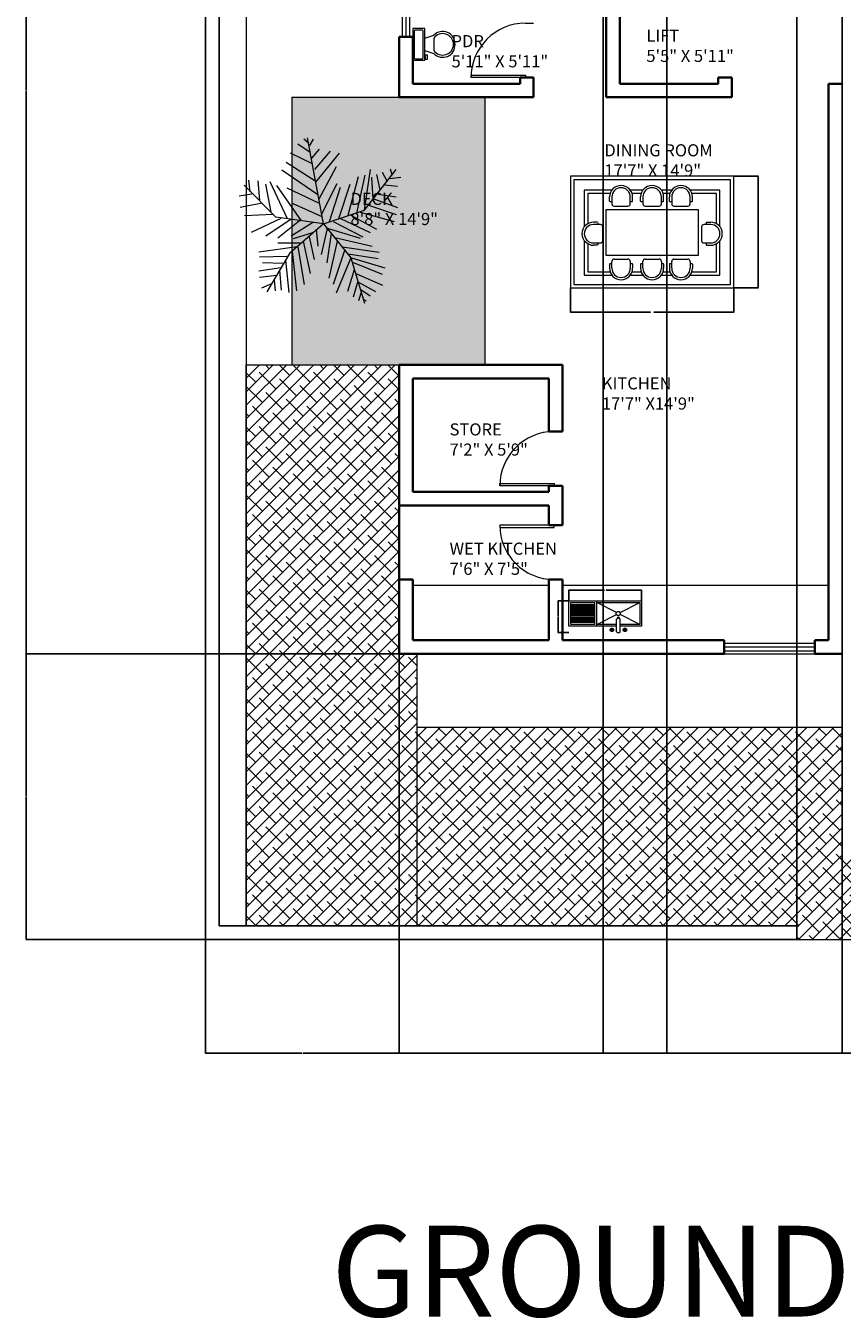
# Model space of a CAD drawing. Units: inches. Extents: x -4843 to -3402, y -164 to 3629.
# Tile 1 of 22: x -4843 to -4303, y -164 to 691. Entities that reach past the tile are written whole.
import ezdxf

# ---------------------------------------------------------------- set-up
doc = ezdxf.new("R2010")
doc.units = ezdxf.units.IN
for name, color, linetype, lineweight in [('A-ANNO-DIMS', 2, 'Continuous', 18), ('A-ANNO-TEXT', 7, 'Continuous', 25), ('A-AREA-IDEN', 2, 'Continuous', 18), ('A-FLOR-CASE', 7, 'Continuous', 18), ('A-FLOR-DECK', 7, 'Continuous', 18), ('C-PROP', 7, 'Continuous', 25), ('C-PVMT', 7, 'Continuous', 18), ('doors', 2, 'Continuous', 18), ('furniture', 6, 'Continuous', 18), ('kitchen', 40, 'Continuous', 18), ('L-PLNT-EDGE', 7, 'Continuous', 18), ('PLANTS', 3, 'Continuous', 13), ('toilets', 5, 'Continuous', 18), ('walls', 7, 'Continuous', 35), ('windows', 1, 'Continuous', 18)]:
    doc.layers.add(name, color=color, linetype=linetype, lineweight=lineweight)
doc.layers.add('A-FLOR-PATT', color=30, linetype='Continuous', lineweight=13, true_color=0xf26722)
doc.layers.add('C-PVMT-PATT', color=9, linetype='Continuous', lineweight=13, true_color=0xc7c8ca)
doc.styles.get("Standard").update_dxf_attribs({"font": 'arial.ttf'})
doc.dimstyles.get("Standard").update_dxf_attribs({"dimtxt": 0.18, "dimasz": 0.18, "dimexe": 0.18, "dimexo": 0.0625, "dimgap": 0.09, "dimtad": 0, "dimtih": 1, "dimtoh": 1, "dimdec": 4, "dimzin": 0, "dimdsep": 46, "dimtxsty": 'Standard', "dimcen": 0.09, "dimadec": 0, "dimazin": 0, "dimtfac": 1, "dimtdec": 4, "dimtofl": 0, "dimtmove": 0, "dimatfit": 3, "dimfxl": 1, "dimtolj": 1, "dimtzin": 0, "dimarcsym": 0})

# ---------------------------------------------------------------- blocks, each defined once
blk = doc.blocks.new('windw 3')
at = {"layer": 'windows'}
for p, q in [((0, 7), (36, 7)), ((0, 4.5), (36, 4.5)), ((0, 2), (36, 2))]:
    blk.add_line(p, q, dxfattribs=at)
for points in [[(0, 0), (0, 9)], [(36, 9), (36, 0)]]:
    blk.add_lwpolyline(points, dxfattribs=at)
blk = doc.blocks.new('window')
at = {"layer": 'windows'}
for p, q in [((0, 7), (60, 7)), ((0, 4.5), (60, 4.5)), ((0, 2), (60, 2))]:
    blk.add_line(p, q, dxfattribs=at)
for points in [[(0, 9), (0, 0)], [(60, 0), (60, 9)]]:
    blk.add_lwpolyline(points, dxfattribs=at)
blk = doc.blocks.new('*U8')
for p, q in [((0, 0), (0, -6)), ((-40, 0), (-40, -6))]:
    blk.add_line(p, q)
blk.add_lwpolyline([(0, 0), (0, 40), (-1.75, 40), (-1.75, 0)], close=True)
blk.add_arc((0, 0), 40, 90, 180)
blk = doc.blocks.new('*U7')
for p, q in [((0, 0), (0, -6)), ((40, 0), (40, -6))]:
    blk.add_line(p, q)
blk.add_lwpolyline([(0, 0), (0, 40), (1.75, 40), (1.75, 0)], close=True)
blk.add_arc((0, 0), 40, 0, 90)
blk = doc.blocks.new('A$C694E1FEF')
for p, q in [((276, 533), (322, 505)), ((313, 542), (284, 496)), ((384, 557), (384, 329)), ((447, 557), (447, 329)), ((505, 514), (559, 524)), ((527, 546), (537, 492)), ((31, 31), (31, 422)), ((31, 422), (385, 243)), ((31, 422), (384, 422)), ((447, 422), (804, 422)), ((804, 422), (451, 243)), ((804, 453), (804, 0)), ((836, 422), (1270, 422)), ((836, 422), (836, 31)), ((836, 390), (1270, 390)), ((1270, 378), (836, 378)), ((836, 359), (1270, 359)), ((1270, 346), (836, 346)), ((836, 327), (1270, 327)), ((1270, 315), (836, 315)), ((836, 296), (1270, 296)), ((1270, 283), (836, 283)), ((836, 264), (1270, 264)), ((1270, 252), (836, 252)), ((836, 233), (1270, 233)), ((1270, 422), (1270, 31)), ((385, 210), (31, 31)), ((804, 31), (31, 31)), ((451, 210), (804, 31)), ((1270, 220), (836, 220)), ((836, 201), (1270, 201)), ((1270, 189), (836, 189)), ((836, 170), (1270, 170)), ((1270, 157), (836, 157)), ((836, 138), (1270, 138)), ((1270, 126), (836, 126)), ((836, 107), (1270, 107)), ((1270, 94), (836, 94)), ((836, 75), (1270, 75)), ((1270, 63), (836, 63)), ((1270, 31), (836, 31))]:
    blk.add_line(p, q)
blk.add_lwpolyline([(447, 453), (1302, 453), (1302, 0), (0, 0), (0, 453), (384, 453)])
for points in [[(329, 519), (329, 527), (321, 541), (307, 549), (290, 549), (276, 541), (268, 527), (268, 511), (276, 497), (290, 489), (307, 489), (321, 497), (329, 511), (329, 519)], [(326, 519), (326, 526), (318, 539), (306, 546), (291, 546), (279, 539), (272, 526), (272, 512), (279, 499), (291, 492), (306, 492), (318, 499), (326, 512), (326, 519)], [(447, 557), (438, 565), (415, 570), (393, 565), (384, 557)], [(562, 519), (562, 527), (554, 541), (540, 549), (524, 549), (510, 541), (502, 527), (502, 511), (510, 497), (524, 489), (540, 489), (554, 497), (562, 511), (562, 519)], [(559, 519), (559, 526), (552, 539), (539, 546), (525, 546), (512, 539), (505, 526), (505, 512), (512, 499), (525, 492), (539, 492), (552, 499), (559, 512), (559, 519)], [(455, 227), (455, 236), (445, 253), (428, 263), (408, 263), (391, 253), (381, 236), (381, 217), (391, 200), (408, 190), (428, 190), (445, 200), (455, 217), (455, 227)], [(384, 329), (389, 321), (406, 312), (425, 312), (442, 321), (447, 329)], [(392, 321), (391, 314), (397, 302), (408, 294), (422, 294), (434, 302), (440, 314), (439, 321)], [(395, 319), (395, 313), (400, 303), (410, 297), (421, 297), (431, 303), (436, 313), (436, 319)]]:
    blk.add_open_spline(points, degree=2)
blk = doc.blocks.new('A$C27801A2F')
for p, q in [((3.55, 2.425), (0, 2.425)), ((0, 2.425), (0, 0)), ((3.475, 2.35), (0.075, 2.35)), ((0.075, 2.35), (0.075, 0.075)), ((3.475, 0.075), (3.475, 2.35)), ((3.55, 0), (3.55, 2.425)), ((0.9, 2.125), (0.3, 2.125)), ((0.3, 2.125), (0.3, 1.325)), ((0.375, 2.05), (0.375, 1.392)), ((0.862, 2.05), (0.375, 2.05)), ((0.85, 1.885), (0.85, 1.975)), ((0.9, 1.975), (0.9, 1.825)), ((1.575, 2.125), (1.3, 2.125)), ((1.3, 1.825), (1.3, 1.975)), ((1.537, 2.05), (1.338, 2.05)), ((1.35, 1.885), (1.35, 1.975)), ((1.525, 1.885), (1.525, 1.975)), ((1.575, 1.975), (1.575, 1.825)), ((2.2, 2.125), (1.975, 2.125)), ((1.975, 1.825), (1.975, 1.975)), ((2.162, 2.05), (2.013, 2.05)), ((2.025, 1.885), (2.025, 1.975)), ((2.15, 1.885), (2.15, 1.975)), ((2.2, 1.975), (2.2, 1.825)), ((3.25, 2.125), (2.6, 2.125)), ((2.6, 1.825), (2.6, 1.975)), ((3.175, 2.05), (2.638, 2.05)), ((2.65, 1.885), (2.65, 1.975)), ((3.175, 1.392), (3.175, 2.05)), ((3.25, 1.325), (3.25, 2.125)), ((0.775, 0.7), (0.775, 1.7)), ((0.775, 1.7), (2.775, 1.7)), ((0.86, 1.875), (0.9, 1.875)), ((0.95, 1.775), (1.25, 1.775)), ((1.3, 1.875), (1.34, 1.875)), ((1.535, 1.875), (1.575, 1.875)), ((1.625, 1.775), (1.925, 1.775)), ((1.975, 1.875), (2.015, 1.875)), ((2.16, 1.875), (2.2, 1.875)), ((2.25, 1.775), (2.55, 1.775)), ((2.6, 1.875), (2.64, 1.875)), ((2.775, 1.7), (2.775, 0.7)), ((0.59, 1.425), (0.5, 1.425)), ((0.6, 1.375), (0.6, 1.415)), ((2.95, 1.415), (2.95, 1.375)), ((2.96, 1.425), (3.05, 1.425)), ((0.65, 1.375), (0.5, 1.375)), ((0.7, 1.025), (0.7, 1.325)), ((2.85, 1.325), (2.85, 1.025)), ((3.05, 1.375), (2.9, 1.375)), ((0.3, 1.025), (0.3, 0.275)), ((0.375, 0.958), (0.375, 0.35)), ((0.5, 0.975), (0.65, 0.975)), ((0.59, 0.925), (0.5, 0.925)), ((0.6, 0.935), (0.6, 0.975)), ((2.9, 0.975), (3.05, 0.975)), ((2.95, 0.975), (2.95, 0.935)), ((2.96, 0.925), (3.05, 0.925)), ((3.175, 0.35), (3.175, 0.958)), ((3.25, 0.275), (3.25, 1.025)), ((2.775, 0.7), (0.775, 0.7)), ((0.9, 0.425), (0.9, 0.575)), ((0.95, 0.625), (1.25, 0.625)), ((1.3, 0.575), (1.3, 0.425)), ((1.575, 0.425), (1.575, 0.575)), ((1.625, 0.625), (1.925, 0.625)), ((1.975, 0.575), (1.975, 0.425)), ((2.2, 0.425), (2.2, 0.575)), ((2.25, 0.625), (2.55, 0.625)), ((2.6, 0.575), (2.6, 0.425)), ((0.375, 0.35), (0.862, 0.35)), ((0.85, 0.515), (0.85, 0.425)), ((0.86, 0.525), (0.9, 0.525)), ((1.3, 0.525), (1.34, 0.525)), ((1.338, 0.35), (1.537, 0.35)), ((1.35, 0.515), (1.35, 0.425)), ((1.525, 0.515), (1.525, 0.425)), ((1.535, 0.525), (1.575, 0.525)), ((1.975, 0.525), (2.015, 0.525)), ((2.013, 0.35), (2.162, 0.35)), ((2.025, 0.515), (2.025, 0.425)), ((2.15, 0.515), (2.15, 0.425)), ((2.16, 0.525), (2.2, 0.525)), ((2.6, 0.525), (2.64, 0.525)), ((2.638, 0.35), (3.175, 0.35)), ((2.65, 0.515), (2.65, 0.425)), ((0, 0), (3.55, 0)), ((0.075, 0.075), (3.475, 0.075)), ((0.3, 0.275), (0.9, 0.275)), ((1.3, 0.275), (1.575, 0.275)), ((1.975, 0.275), (2.2, 0.275)), ((2.6, 0.275), (3.25, 0.275))]:
    blk.add_line(p, q)
for centre, radius, start, end in [((1.1, 1.975), 0.25, 0, 180), ((1.1, 1.975), 0.2, 0.0001, 179.9999), ((1.775, 1.975), 0.25, 0, 180), ((1.775, 1.975), 0.2, 0.0001, 179.9999), ((2.4, 1.975), 0.25, 0, 180), ((2.4, 1.975), 0.2, 0.0001, 179.9999), ((0.86, 1.885), 0.01, 180, 270), ((0.95, 1.825), 0.05, 180, 270), ((1.25, 1.825), 0.05, 270, 0), ((1.34, 1.885), 0.01, 270, 0), ((1.535, 1.885), 0.01, 180, 270), ((1.625, 1.825), 0.05, 180, 270), ((1.925, 1.825), 0.05, 270, 0), ((2.015, 1.885), 0.01, 270, 0), ((2.16, 1.885), 0.01, 180, 270), ((2.25, 1.825), 0.05, 180, 270), ((2.55, 1.825), 0.05, 270, 0), ((2.64, 1.885), 0.01, 270, 0), ((0.5, 1.175), 0.25, 90, 270), ((2.96, 1.415), 0.01, 90, 180), ((3.05, 1.175), 0.25, 270, 90), ((0.5, 1.175), 0.2, 90.0001, 269.9999), ((0.65, 1.325), 0.05, 0, 90), ((2.9, 1.325), 0.05, 90, 180), ((3.05, 1.175), 0.2, 270.0001, 89.9999), ((0.65, 1.025), 0.05, 270, 0), ((2.9, 1.025), 0.05, 180, 270), ((2.96, 0.935), 0.01, 180, 270), ((0.95, 0.575), 0.05, 90, 180), ((1.25, 0.575), 0.05, 0, 90), ((1.625, 0.575), 0.05, 90, 180), ((1.925, 0.575), 0.05, 0, 90), ((2.25, 0.575), 0.05, 90, 180), ((2.55, 0.575), 0.05, 0, 90), ((0.86, 0.515), 0.01, 90, 180), ((1.1, 0.425), 0.25, 180, 0), ((1.1, 0.425), 0.2, 180.0001, 359.9999), ((1.34, 0.515), 0.01, 0, 90), ((1.535, 0.515), 0.01, 90, 180), ((1.775, 0.425), 0.25, 180, 0), ((1.775, 0.425), 0.2, 180.0001, 359.9999), ((2.015, 0.515), 0.01, 0, 90), ((2.16, 0.515), 0.01, 90, 180), ((2.4, 0.425), 0.25, 180, 0), ((2.4, 0.425), 0.2, 180.0001, 359.9999), ((2.64, 0.515), 0.01, 0, 90)]:
    blk.add_arc(centre, radius, start, end)
blk = doc.blocks.new('*U31')
for p, q in [((-254, -215.9), (-203.2, -215.9)), ((-254, -241.3), (-254, -215.9)), ((-203.2, -215.9), (-203.2, -203.2)), ((-177.8, -203.2), (-177.8, -241.3)), ((-101.6, -203.2), (-152.4, -355.6)), ((101.6, -203.2), (152.4, -355.6)), ((241.3, -152.4), (241.3, -50.8)), ((-177.8, -241.3), (-254, -241.3)), ((101.6, -355.6), (-101.6, -355.6))]:
    blk.add_line(p, q)
blk.add_lwpolyline([(266.7, -203.2), (266.7, 0), (-266.7, 0), (-266.7, -203.2)], close=True)
for points in [[(-241.3, -50.8), (-241.3, -152.4)], [(215.9, -25.4), (-215.9, -25.4)], [(-215.9, -177.8), (215.9, -177.8)]]:
    blk.add_lwpolyline(points)
for centre, radius, start, end in [((-219.075, -47.625), 22.45064, 81.8699, 188.1301), ((-219.075, -155.575), 22.45064, 171.869898, 278.1301), ((219.075, -47.625), 22.45064, 351.8699, 98.1301), ((219.075, -155.575), 22.45064, 261.8699, 8.1301), ((-12.12088, -505.93752), 205.61935, 133.01722, 273.38), ((0.94996, -504.77674), 181.02486, 124.50543, 269.7), ((-0.94742, -504.77674), 181.02486, 270.3, 55.4946), ((12.12342, -505.93752), 205.61935, 266.62, 46.9828)]:
    blk.add_arc(centre, radius, start, end)
blk = doc.blocks.new('*U33')
for p, q in [((-221.9198, 1197.3052), (-433.5526, 1338.8594)), ((-258.7244, 1362.456), (-332.3336, 1421.4348)), ((0, 0), (-266.7, 1447.8)), ((-231.1146, 1315.2628), (-166.7002, 1421.4348)), ((-185.1152, 1008.5578), (-553.1612, 1185.4942)), ((-194.31, 1102.9442), (-65.4812, 1256.284)), ((-148.3106, 914.1968), (118.5418, 1220.9018)), ((-129.8956, 701.8528), (265.7602, 1185.4942)), ((-93.091, 489.5342), (-700.3796, 902.3858)), ((-129.8956, 713.6638), (-626.7704, 1032.1544)), ((-74.7014, 418.7444), (219.7608, 961.39)), ((685.8, 228.6), (1219.2, 914.4)), ((689.0258, 230.0224), (790.2448, 914.1968)), ((1121.4862, 925.9824), (1149.0706, 831.6214)), ((-1234.059, 536.7274), (-1252.4486, 737.2604)), ((-1105.2302, 725.4494), (-1077.6458, 395.1732)), ((-976.4268, 666.4706), (-884.4026, 194.6402)), ((-902.8176, 713.6638), (-617.5756, 100.2538)), ((-28.6766, 171.0436), (228.9556, 678.2816)), ((256.5654, 88.4682), (449.7832, 666.4706)), ((412.9786, 147.447), (587.8068, 796.2392)), ((560.197, 182.8292), (698.2206, 819.8358)), ((808.6344, 784.4282), (827.0494, 418.7444)), ((891.4384, 831.6214), (946.658, 572.1096)), ((983.4626, 867.0036), (1066.2666, 725.4494)), ((1029.462, 654.685), (1241.0948, 631.0884)), ((1112.2914, 760.8316), (1296.3144, 784.4282)), ((-1206.4492, 501.3198), (-1418.082, 465.9376)), ((-800.1, 114.3), (-1333.5, 647.7)), ((-369.1382, 53.086), (-783.1836, 642.874)), ((-617.5756, 607.4918), (-74.7014, 347.98)), ((100.1268, 41.275), (284.1498, 619.2774)), ((919.0482, 501.3198), (1222.6798, 454.152)), ((-1031.621, 347.98), (-1399.667, 277.1902)), ((-525.5514, 347.98), (-28.6766, 123.8504)), ((0, 0), (685.8, 228.6)), ((753.4148, 312.5978), (1222.6798, 159.2326)), ((845.439, 418.7444), (1241.0948, 277.1902)), ((-847.598, 159.2326), (-1326.0578, 135.636)), ((-718.7946, 88.4682), (-1215.644, -147.447)), ((-543.9664, 76.6572), (-967.2066, -206.4512)), ((0, 0), (-800.1, 114.3)), ((-405.9428, 53.086), (-764.794, -241.8334)), ((0, 0), (-571.5, -495.3)), ((-166.7002, 29.4894), (-543.9664, -206.4512)), ((0, 0), (457.2, -571.5)), ((164.5412, 41.275), (661.416, -218.2368)), ((284.1498, 88.4682), (781.0246, -147.447)), ((458.978, 147.447), (891.4384, -88.4682)), ((615.4166, 194.6402), (1185.8752, 41.275)), ((-166.7002, -147.447), (-507.1618, -253.619)), ((-120.7008, -88.4682), (-93.091, -371.5766)), ((63.3222, -76.6826), (-37.8714, -513.1308)), ((44.9326, -64.897), (615.4166, -241.8334)), ((127.7366, -159.258), (54.1274, -654.685)), ((-442.7474, -383.3876), (-1086.8406, -477.7486)), ((-387.5278, -324.4088), (-764.794, -324.4088)), ((-433.5526, -383.3876), (-323.1134, -1020.3688)), ((-341.5284, -289.0012), (-221.9198, -831.6214)), ((-240.3094, -218.2368), (-157.5054, -595.7062)), ((228.9556, -289.0012), (90.932, -914.1968)), ((357.759, -430.5554), (164.5412, -1020.3688)), ((192.151, -230.0224), (817.8292, -371.5766)), ((311.7596, -383.3876), (937.4378, -477.7486)), ((-617.5756, -548.5384), (-1077.6458, -560.324)), ((-571.5, -495.3), (-952.5, -1143)), ((-635.9652, -607.5172), (-580.771, -1150.1374)), ((-525.5514, -465.963), (-451.9422, -1126.5408)), ((458.978, -572.1096), (210.5406, -1161.923)), ((412.9786, -501.3452), (919.0482, -583.9206)), ((457.2, -571.5), (685.8, -1333.5)), ((468.1982, -572.1096), (1029.462, -737.2604)), ((486.5878, -642.8994), (983.4626, -843.4324)), ((-718.7946, -737.2604), (-1086.8406, -796.2392)), ((-783.1836, -867.029), (-1077.6458, -902.4112)), ((-681.9646, -666.496), (-1022.4262, -654.685)), ((-737.1842, -784.4536), (-709.5744, -1114.7298)), ((514.1976, -772.6426), (403.7838, -1138.3264)), ((541.8074, -831.6214), (992.6574, -1032.1544)), ((-875.2078, -1008.5832), (-1040.8412, -1079.3476)), ((-829.2084, -937.7934), (-810.7934, -1126.5408)), ((578.612, -961.39), (495.7826, -1232.7128)), ((578.612, -973.1756), (873.0488, -1138.3264)), ((624.6114, -1161.923), (587.8068, -1291.6916)), ((624.6114, -1102.9442), (781.0246, -1209.1162)), ((679.8056, -1268.095), (716.6102, -1291.6916))]:
    blk.add_line(p, q)
blk = doc.blocks.new('*D52')
at = {"layer": 'A-ANNO-DIMS', "color": 0, "lineweight": -2, "transparency": 16777216}
for p, q in [((-4483.42, 310.32), (-4483.42, 317.64)), ((-4483.24, 317.46), (-4459.96, 317.46)), ((-4435.6, 317.46), (-4458.87, 317.46)), ((-4435.42, 310.32), (-4435.42, 317.64))]:
    blk.add_line(p, q, dxfattribs=at)
at = {"layer": 'A-ANNO-DIMS', "color": 0, "transparency": 16777216}
for points in [[(-4483.24, 317.49), (-4483.24, 317.43), (-4483.42, 317.46)], [(-4435.6, 317.49), (-4435.6, 317.43), (-4435.42, 317.46)]]:
    blk.add_solid(points, dxfattribs=at)
at = {"layer": 'Defpoints', "color": 0, "transparency": 16777216}
for p in [(-4483.42, 317.46), (-4483.42, 310.26), (-4435.42, 310.26)]:
    blk.add_point(p, dxfattribs=at)
at = {"layer": 'A-ANNO-DIMS', "color": 0, "transparency": 16777216, "insert": (-4459.42, 317.46), "char_height": 0.18, "attachment_point": 5}
blk.add_mtext('\\A1;SINK 48', dxfattribs=at)
blk = doc.blocks.new('*D53')
at = {"layer": 'A-ANNO-DIMS', "color": 0, "lineweight": -2, "transparency": 16777216}
for p, q in [((-4483.48, 310.26), (-4490.8, 310.26)), ((-4490.62, 310.08), (-4490.62, 299.95)), ((-4490.62, 289.47), (-4490.62, 299.59)), ((-4483.48, 289.29), (-4490.8, 289.29))]:
    blk.add_line(p, q, dxfattribs=at)
at = {"layer": 'A-ANNO-DIMS', "color": 0, "transparency": 16777216}
for points in [[(-4490.65, 310.08), (-4490.59, 310.08), (-4490.62, 310.26)], [(-4490.65, 289.47), (-4490.59, 289.47), (-4490.62, 289.29)]]:
    blk.add_solid(points, dxfattribs=at)
at = {"layer": 'Defpoints', "color": 0, "transparency": 16777216}
for p in [(-4483.42, 310.26), (-4490.62, 289.29), (-4483.42, 289.29)]:
    blk.add_point(p, dxfattribs=at)
at = {"layer": 'A-ANNO-DIMS', "color": 0, "transparency": 16777216, "insert": (-4490.62, 299.77), "char_height": 0.18, "attachment_point": 5}
blk.add_mtext('\\A1;21', dxfattribs=at)
blk = doc.blocks.new('*D56')
at = {"layer": 'A-ANNO-DIMS', "color": 0, "lineweight": -2, "transparency": 16777216}
for p, q in [((-4482.43, 517.3), (-4482.43, 500.98)), ((-4374.43, 517.3), (-4374.43, 500.98)), ((-4482.25, 501.16), (-4429.47, 501.16)), ((-4374.61, 501.16), (-4427.39, 501.16))]:
    blk.add_line(p, q, dxfattribs=at)
at = {"layer": 'A-ANNO-DIMS', "color": 0, "transparency": 16777216}
for points in [[(-4482.25, 501.19), (-4482.25, 501.13), (-4482.43, 501.16)], [(-4374.61, 501.19), (-4374.61, 501.13), (-4374.43, 501.16)]]:
    blk.add_solid(points, dxfattribs=at)
at = {"layer": 'Defpoints', "color": 0, "transparency": 16777216}
for p in [(-4482.43, 517.36), (-4374.43, 517.36), (-4374.43, 501.16)]:
    blk.add_point(p, dxfattribs=at)
at = {"layer": 'A-ANNO-DIMS', "color": 0, "transparency": 16777216, "insert": (-4428.43, 501.16), "char_height": 0.18, "attachment_point": 5}
blk.add_mtext('\\A1;DINING SET 108', dxfattribs=at)
blk = doc.blocks.new('*D57')
at = {"layer": 'A-ANNO-DIMS', "color": 0, "lineweight": -2, "transparency": 16777216}
for p, q in [((-4374.37, 591.14), (-4358.05, 591.14)), ((-4358.23, 590.96), (-4358.23, 554.43)), ((-4358.23, 517.54), (-4358.23, 554.07)), ((-4374.37, 517.36), (-4358.05, 517.36))]:
    blk.add_line(p, q, dxfattribs=at)
at = {"layer": 'A-ANNO-DIMS', "color": 0, "transparency": 16777216}
for points in [[(-4358.26, 590.96), (-4358.2, 590.96), (-4358.23, 591.14)], [(-4358.26, 517.54), (-4358.2, 517.54), (-4358.23, 517.36)]]:
    blk.add_solid(points, dxfattribs=at)
at = {"layer": 'Defpoints', "color": 0, "transparency": 16777216}
for p in [(-4374.43, 591.14), (-4358.23, 591.14), (-4374.43, 517.36)]:
    blk.add_point(p, dxfattribs=at)
at = {"layer": 'A-ANNO-DIMS', "color": 0, "transparency": 16777216, "insert": (-4358.23, 554.25), "char_height": 0.18, "attachment_point": 5}
blk.add_mtext('\\A1;74', dxfattribs=at)
blk = doc.blocks.new('*D62')
at = {"layer": 'A-ANNO-DIMS', "color": 0, "lineweight": -2, "transparency": 16777216}
for p, q in [((-4595.78, 275.29), (-4595.78, 10.92)), ((-4302.78, 275.29), (-4302.78, 10.92)), ((-4595.6, 11.1), (-4449.57, 11.1)), ((-4302.96, 11.1), (-4448.99, 11.1))]:
    blk.add_line(p, q, dxfattribs=at)
at = {"layer": 'A-ANNO-DIMS', "color": 0, "transparency": 16777216}
for points in [[(-4595.6, 11.13), (-4595.6, 11.07), (-4595.78, 11.1)], [(-4302.96, 11.13), (-4302.96, 11.07), (-4302.78, 11.1)]]:
    blk.add_solid(points, dxfattribs=at)
at = {"layer": 'Defpoints', "color": 0, "transparency": 16777216}
for p in [(-4595.78, 275.35), (-4302.78, 275.35), (-4302.78, 11.1)]:
    blk.add_point(p, dxfattribs=at)
at = {"layer": 'A-ANNO-DIMS', "color": 0, "transparency": 16777216, "insert": (-4449.28, 11.1), "char_height": 0.18, "attachment_point": 5}
blk.add_mtext('\\A1;293', dxfattribs=at)
blk = doc.blocks.new('*D63')
at = {"layer": 'A-ANNO-DIMS', "color": 0, "lineweight": -2, "transparency": 16777216}
for p, q in [((-4083.78, 457.29), (-4083.78, 10.92)), ((-4302.78, 275.29), (-4302.78, 10.92)), ((-4302.6, 11.1), (-4193.57, 11.1)), ((-4083.96, 11.1), (-4192.99, 11.1))]:
    blk.add_line(p, q, dxfattribs=at)
at = {"layer": 'A-ANNO-DIMS', "color": 0, "transparency": 16777216}
for points in [[(-4302.6, 11.13), (-4302.6, 11.07), (-4302.78, 11.1)], [(-4083.96, 11.13), (-4083.96, 11.07), (-4083.78, 11.1)]]:
    blk.add_solid(points, dxfattribs=at)
at = {"layer": 'Defpoints', "color": 0, "transparency": 16777216}
for p in [(-4083.78, 457.35), (-4302.78, 275.35), (-4083.78, 11.1)]:
    blk.add_point(p, dxfattribs=at)
at = {"layer": 'A-ANNO-DIMS', "color": 0, "transparency": 16777216, "insert": (-4193.28, 11.1), "char_height": 0.18, "attachment_point": 5}
blk.add_mtext('\\A1;219', dxfattribs=at)
blk = doc.blocks.new('*D64')
at = {"layer": 'A-ANNO-DIMS', "color": 0, "lineweight": -2, "transparency": 16777216}
for p, q in [((-4595.85, 1020.35), (-4842.55, 1020.35)), ((-4842.37, 1020.17), (-4842.37, 648.04)), ((-4842.37, 275.53), (-4842.37, 647.67)), ((-4595.85, 275.35), (-4842.55, 275.35))]:
    blk.add_line(p, q, dxfattribs=at)
at = {"layer": 'A-ANNO-DIMS', "color": 0, "transparency": 16777216}
for points in [[(-4842.4, 1020.17), (-4842.34, 1020.17), (-4842.37, 1020.35)], [(-4842.4, 275.53), (-4842.34, 275.53), (-4842.37, 275.35)]]:
    blk.add_solid(points, dxfattribs=at)
at = {"layer": 'Defpoints', "color": 0, "transparency": 16777216}
for p in [(-4595.78, 1020.35), (-4842.37, 275.35), (-4595.78, 275.35)]:
    blk.add_point(p, dxfattribs=at)
at = {"layer": 'A-ANNO-DIMS', "color": 0, "transparency": 16777216, "insert": (-4842.37, 647.85), "char_height": 0.18, "attachment_point": 5}
blk.add_mtext('\\A1;745', dxfattribs=at)
blk = doc.blocks.new('*D65')
at = {"layer": 'A-ANNO-DIMS', "color": 0, "lineweight": -2, "transparency": 16777216}
for p, q in [((-4595.78, 275.29), (-4595.78, 10.92)), ((-4723.78, 86.29), (-4723.78, 10.92)), ((-4723.6, 11.1), (-4660.06, 11.1)), ((-4595.96, 11.1), (-4659.5, 11.1))]:
    blk.add_line(p, q, dxfattribs=at)
at = {"layer": 'A-ANNO-DIMS', "color": 0, "transparency": 16777216}
for points in [[(-4723.6, 11.13), (-4723.6, 11.07), (-4723.78, 11.1)], [(-4595.96, 11.13), (-4595.96, 11.07), (-4595.78, 11.1)]]:
    blk.add_solid(points, dxfattribs=at)
at = {"layer": 'Defpoints', "color": 0, "transparency": 16777216}
for p in [(-4595.78, 275.35), (-4723.78, 86.35), (-4595.78, 11.1)]:
    blk.add_point(p, dxfattribs=at)
at = {"layer": 'A-ANNO-DIMS', "color": 0, "transparency": 16777216, "insert": (-4659.78, 11.1), "char_height": 0.18, "attachment_point": 5}
blk.add_mtext('\\A1;128', dxfattribs=at)
blk = doc.blocks.new('*D67')
at = {"layer": 'A-ANNO-DIMS', "color": 0, "lineweight": -2, "transparency": 16777216}
for p, q in [((-4595.85, 275.35), (-4842.55, 275.35)), ((-4842.37, 275.17), (-4842.37, 181.04)), ((-4842.37, 86.53), (-4842.37, 180.67)), ((-4723.85, 86.35), (-4842.55, 86.35))]:
    blk.add_line(p, q, dxfattribs=at)
at = {"layer": 'A-ANNO-DIMS', "color": 0, "transparency": 16777216}
for points in [[(-4842.4, 275.17), (-4842.34, 275.17), (-4842.37, 275.35)], [(-4842.4, 86.53), (-4842.34, 86.53), (-4842.37, 86.35)]]:
    blk.add_solid(points, dxfattribs=at)
at = {"layer": 'Defpoints', "color": 0, "transparency": 16777216}
for p in [(-4595.78, 275.35), (-4842.37, 86.35), (-4723.78, 86.35)]:
    blk.add_point(p, dxfattribs=at)
at = {"layer": 'A-ANNO-DIMS', "color": 0, "transparency": 16777216, "insert": (-4842.37, 180.85), "char_height": 0.18, "attachment_point": 5}
blk.add_mtext('\\A1;189', dxfattribs=at)
blk = doc.blocks.new('*D75')
at = {"layer": 'A-ANNO-DIMS', "color": 0, "lineweight": -2, "transparency": 16777216}
for p, q in [((-4460.78, 819.29), (-4460.78, 10.92)), ((-4418.78, 819.29), (-4418.78, 10.92)), ((-4460.6, 11.1), (-4440, 11.1)), ((-4418.96, 11.1), (-4439.56, 11.1))]:
    blk.add_line(p, q, dxfattribs=at)
at = {"layer": 'A-ANNO-DIMS', "color": 0, "transparency": 16777216}
for points in [[(-4460.6, 11.13), (-4460.6, 11.07), (-4460.78, 11.1)], [(-4418.96, 11.13), (-4418.96, 11.07), (-4418.78, 11.1)]]:
    blk.add_solid(points, dxfattribs=at)
at = {"layer": 'Defpoints', "color": 0, "transparency": 16777216}
for p in [(-4460.78, 819.35), (-4418.78, 819.35), (-4418.78, 11.1)]:
    blk.add_point(p, dxfattribs=at)
at = {"layer": 'A-ANNO-DIMS', "color": 0, "transparency": 16777216, "insert": (-4439.78, 11.1), "char_height": 0.18, "attachment_point": 5}
blk.add_mtext('\\A1;42', dxfattribs=at)
blk = doc.blocks.new('*D76')
at = {"layer": 'A-ANNO-DIMS', "color": 0, "lineweight": -2, "transparency": 16777216}
for p, q in [((-4418.78, 819.29), (-4418.78, 10.92)), ((-4302.78, 819.29), (-4302.78, 10.92)), ((-4418.6, 11.1), (-4361.06, 11.1)), ((-4302.96, 11.1), (-4360.5, 11.1))]:
    blk.add_line(p, q, dxfattribs=at)
at = {"layer": 'A-ANNO-DIMS', "color": 0, "transparency": 16777216}
for points in [[(-4418.6, 11.13), (-4418.6, 11.07), (-4418.78, 11.1)], [(-4302.96, 11.13), (-4302.96, 11.07), (-4302.78, 11.1)]]:
    blk.add_solid(points, dxfattribs=at)
at = {"layer": 'Defpoints', "color": 0, "transparency": 16777216}
for p in [(-4418.78, 819.35), (-4302.78, 819.35), (-4302.78, 11.1)]:
    blk.add_point(p, dxfattribs=at)
at = {"layer": 'A-ANNO-DIMS', "color": 0, "transparency": 16777216, "insert": (-4360.78, 11.1), "char_height": 0.18, "attachment_point": 5}
blk.add_mtext('\\A1;116', dxfattribs=at)
blk = doc.blocks.new('*D81')
at = {"layer": 'A-ANNO-DIMS', "color": 0, "lineweight": -2, "transparency": 16777216}
for p, q in [((-4332.78, 86.42), (-4332.78, 1392.95)), ((-4332.6, 1392.77), (-4168.61, 1392.77)), ((-4003.86, 1392.77), (-4167.86, 1392.77)), ((-4003.68, 86.42), (-4003.68, 1392.95))]:
    blk.add_line(p, q, dxfattribs=at)
at = {"layer": 'A-ANNO-DIMS', "color": 0, "transparency": 16777216}
for points in [[(-4332.6, 1392.8), (-4332.6, 1392.74), (-4332.78, 1392.77)], [(-4003.86, 1392.8), (-4003.86, 1392.74), (-4003.68, 1392.77)]]:
    blk.add_solid(points, dxfattribs=at)
at = {"layer": 'Defpoints', "color": 0, "transparency": 16777216}
for p in [(-4003.68, 1392.77), (-4332.78, 86.35), (-4003.68, 86.35)]:
    blk.add_point(p, dxfattribs=at)
at = {"layer": 'A-ANNO-DIMS', "color": 0, "transparency": 16777216, "insert": (-4168.23, 1392.77), "char_height": 0.18, "attachment_point": 5}
blk.add_mtext('\\A1;329.1', dxfattribs=at)

msp = doc.modelspace()

# ---------------------------------------------------------------- hatches: boundary and pattern name
at = {"layer": 'A-FLOR-PATT', "transparency": 33554472}
h = msp.add_hatch(color=256, dxfattribs=at)
h.dxf.hatch_style = 1
h.paths.add_polyline_path([(-4538.62, 643.09), (-4595.62, 643.09), (-4666.62, 643.09), (-4666.62, 466.09), (-4595.62, 466.09), (-4538.62, 466.09)])
h.paths.add_polyline_path([(-3998.62, 888.09), (-4083.62, 888.09), (-4140.62, 888.09), (-4140.62, 652.09), (-4132.62, 652.09), (-4132.62, 650.09), (-4096.62, 650.09), (-4096.62, 652.09), (-4083.62, 652.09), (-3998.62, 652.09)])
at = {"layer": 'C-PVMT-PATT'}
h = msp.add_hatch(dxfattribs=at)
h.set_pattern_fill('ANSI38', color=256, scale=2)
h.set_pattern_definition([(45, (-7766.296, -1992.247), (-4.490128, 4.490128), []), (135, (-7766.296, -1992.247), (-13.470384, 4.490128), [15.875, -9.525])])
h.paths.add_polyline_path([(-4583.98, 275.35), (-4595.78, 275.35), (-4595.78, 324.35), (-4595.78, 373.35), (-4595.78, 466.35), (-4696.78, 466.35), (-4696.78, 95.35), (-4583.98, 95.35), (-4583.98, 226.6)])
h.paths.add_polyline_path([(-4302.78, 226.6), (-4583.98, 226.6), (-4583.98, 95.35), (-4332.78, 95.35), (-4332.78, 86.35), (-4003.68, 86.35), (-4003.68, 95.35), (-3978.78, 95.35), (-3978.78, 457.35), (-4003.68, 457.35), (-4003.68, 139.54), (-4302.78, 139.54)])

# ---------------------------------------------------------------- linework, layer by layer
at = {"layer": 'A-FLOR-CASE'}
for p, q in [((-4496.78, 320.35), (-4586.78, 320.35)), ((-4311.78, 320.35), (-4487.78, 320.35))]:
    msp.add_line(p, q, dxfattribs=at)
at = {"layer": 'A-FLOR-DECK'}
for p, q in [((-4666.78, 643.35), (-4666.78, 466.35)), ((-4666.78, 643.35), (-4595.78, 643.35)), ((-4538.78, 466.35), (-4538.78, 643.35)), ((-4538.78, 466.35), (-4538.78, 643.35)), ((-4666.78, 466.35), (-4595.78, 466.35))]:
    msp.add_line(p, q, dxfattribs=at)
at = {"layer": 'C-PROP'}
for p, q in [((-4723.78, 1149.35), (-4723.78, 86.35)), ((-4714.78, 1140.35), (-4714.78, 95.35)), ((-4714.78, 95.35), (-4332.78, 95.35)), ((-4332.78, 86.35), (-4332.78, 95.35)), ((-4723.78, 86.35), (-4332.78, 86.35))]:
    msp.add_line(p, q, dxfattribs=at)
at = {"layer": 'C-PVMT'}
for p, q in [((-4583.98, 226.6), (-4583.98, 95.35)), ((-4332.78, 86.35), (-4003.68, 86.35))]:
    msp.add_line(p, q, dxfattribs=at)
for points in [[(-4583.98, 95.35), (-4696.78, 95.35), (-4696.78, 466.35), (-4583.98, 466.35)], [(-4583.98, 275.35), (-4583.98, 226.6)], [(-4583.63, 275.35), (-4302.78, 275.35), (-4302.78, 226.6), (-4583.98, 226.6)]]:
    msp.add_lwpolyline(points, dxfattribs=at)
at = {"layer": 'L-PLNT-EDGE'}
msp.add_line((-4696.78, 1116.35), (-4696.78, 95.35), dxfattribs=at)
at = {"layer": 'walls'}
for p, q in [((-4458.78, 723.35), (-4458.78, 643.35)), ((-4449.78, 723.35), (-4449.78, 652.35)), ((-4595.78, 683.35), (-4595.78, 643.35)), ((-4586.78, 683.35), (-4586.78, 652.35)), ((-4586.78, 652.35), (-4515.78, 652.35)), ((-4515.78, 656.35), (-4515.78, 652.35)), ((-4506.78, 656.35), (-4506.78, 643.35)), ((-4449.78, 652.35), (-4384.78, 652.35)), ((-4384.78, 656.35), (-4384.78, 652.35)), ((-4375.78, 656.35), (-4375.78, 643.35)), ((-4311.78, 652.35), (-4311.78, 284.35)), ((-4302.78, 652.35), (-4311.78, 652.35)), ((-4595.78, 643.35), (-4506.78, 643.35)), ((-4458.78, 643.35), (-4375.78, 643.35)), ((-4487.78, 466.35), (-4595.78, 466.35)), ((-4595.78, 466.35), (-4595.78, 373.35)), ((-4487.78, 422.35), (-4487.78, 466.35)), ((-4496.78, 457.35), (-4586.78, 457.35)), ((-4586.78, 457.35), (-4586.78, 382.35)), ((-4496.78, 422.35), (-4496.78, 457.35)), ((-4496.78, 382.35), (-4496.78, 386.35)), ((-4487.78, 360.35), (-4487.78, 386.35)), ((-4586.78, 382.35), (-4496.78, 382.35)), ((-4586.78, 373.35), (-4595.78, 373.35)), ((-4595.78, 324.35), (-4595.78, 373.35)), ((-4586.78, 373.35), (-4496.78, 373.35)), ((-4496.78, 360.35), (-4496.78, 373.35)), ((-4586.78, 324.35), (-4595.78, 324.35)), ((-4595.78, 324.35), (-4595.78, 275.35)), ((-4586.78, 324.35), (-4586.78, 284.35)), ((-4496.78, 284.35), (-4496.78, 324.35)), ((-4487.78, 284.35), (-4487.78, 324.35)), ((-4496.78, 284.35), (-4586.78, 284.35)), ((-4380.78, 284.35), (-4487.78, 284.35)), ((-4380.78, 284.35), (-4487.78, 284.35)), ((-4380.78, 275.35), (-4380.78, 284.35)), ((-4311.78, 284.35), (-4320.78, 284.35)), ((-4311.78, 284.35), (-4320.78, 284.35)), ((-4320.78, 275.35), (-4320.78, 284.35)), ((-4380.78, 275.35), (-4595.78, 275.35)), ((-4302.78, 275.35), (-4320.78, 275.35))]:
    msp.add_line(p, q, dxfattribs=at)
for points in [[(-4586.78, 683.35), (-4595.78, 683.35)], [(-4506.78, 656.35), (-4515.78, 656.35)], [(-4375.78, 656.35), (-4384.78, 656.35)], [(-4496.78, 422.35), (-4487.78, 422.35)], [(-4487.78, 386.35), (-4496.78, 386.35)], [(-4496.78, 360.35), (-4487.78, 360.35)], [(-4487.78, 324.35), (-4496.78, 324.35)]]:
    msp.add_lwpolyline(points, dxfattribs=at)

# ---------------------------------------------------------------- block references
at = {"layer": 'doors', "xscale": 0.9, "yscale": 0.9, "zscale": 0.9, "rotation": 90}
for name, p in [('*U7', (-4512.18, 656.35)), ('*U7', (-4493.18, 386.35)), ('*U8', (-4493.18, 360.35))]:
    msp.add_blockref(name, p, dxfattribs=at)
at = {"layer": 'furniture', "xscale": 30.42253521127383, "yscale": 30.42253521127383, "zscale": 30.42253521127383}
msp.add_blockref('A$C27801A2F', (-4482.43, 517.36), dxfattribs=at)
at = {"layer": 'kitchen', "xscale": 0.0368764537023914, "yscale": 0.0368764537023914, "zscale": 0.0368764537023914, "rotation": 180}
msp.add_blockref('A$C694E1FEF', (-4435.42, 310.26), dxfattribs=at)
at = {"layer": 'PLANTS', "xscale": 0.0393700787401575, "yscale": 0.0393700787401575, "zscale": 0.0393700787401575}
msp.add_blockref('*U33', (-4645.74, 559.62), dxfattribs=at)
at = {"layer": 'toilets', "xscale": 0.0393700787401575, "yscale": 0.0393700787401575, "zscale": 0.0393700787401575, "rotation": 90}
msp.add_blockref('*U31', (-4586.78, 678.35), dxfattribs=at)
at = {"layer": 'windows', "rotation": 270}
msp.add_blockref('windw 3', (-4595.78, 719.35), dxfattribs=at)
at = {"layer": 'windows'}
msp.add_blockref('window', (-4380.78, 275.35), dxfattribs=at)

# ---------------------------------------------------------------- texts
at = {"layer": 'A-ANNO-TEXT'}
msp.add_text('GROUND FLOOR', height=60, dxfattribs=at).set_placement((-4640.63, -163.06))
at = {"layer": 'A-AREA-IDEN', "char_height": 8, "attachment_point": 1}
for s, width, heights, insert in [('PDR\\P5\'11" X 5\'11"', 66.873, [0], (-4561.07, 684.49)), ('LIFT\\P5\'5" X 5\'11"', 66.873, [0], (-4432.24, 688.07)), ('DINING ROOM\\P17\'7" X 14\'9"', 98.9475, [0], (-4459.99, 612.29)), ('DECK\\P8\'8" X 14\'9"', 66.873, [0], (-4627.89, 580.18)), ('KITCHEN \\P17\'7" X14\'9"', 66.873, [0], (-4461.65, 458.14)), ('STORE \\P7\'2" X 5\'9"', 66.873, [0], (-4562.37, 427.68)), ('WET KITCHEN\\P7\'6" X 7\'5"', 139.7591, [37.02], (-4562.37, 348.82))]:
    msp.add_mtext_dynamic_manual_height_columns(s, width=width, gutter_width=60, heights=heights, dxfattribs=dict(at, insert=insert))

# ---------------------------------------------------------------- dimensions: what is measured, and where the dimension line sits
at = {"layer": 'A-ANNO-DIMS'}
for base, p1, p2, override, picture, middle in [((-4003.68, 1392.77), (-4332.78, 86.35), (-4003.68, 86.35), {"dimdec": 1, "dimlfac": 1, "dimrnd": 0, "dimzin": 0, "dimdsep": 46, "dimlunit": 2}, '*D81', (-4168.23, 1392.77)), ((-4418.78, 11.1), (-4460.78, 819.35), (-4418.78, 819.35), {"dimdec": 0, "dimlfac": 1, "dimrnd": 0, "dimzin": 0, "dimdsep": 46, "dimlunit": 2}, '*D75', (-4439.78, 11.1)), ((-4302.78, 11.1), (-4418.78, 819.35), (-4302.78, 819.35), {"dimdec": 0, "dimlfac": 1, "dimrnd": 0, "dimzin": 0, "dimdsep": 46, "dimlunit": 2}, '*D76', (-4360.78, 11.1)), ((-4083.78, 11.1), (-4302.78, 275.35), (-4083.78, 457.35), {"dimdec": 0, "dimlfac": 1, "dimrnd": 0, "dimzin": 0, "dimdsep": 46, "dimlunit": 2}, '*D63', (-4193.28, 11.1)), ((-4595.78, 11.1), (-4723.78, 86.35), (-4595.78, 275.35), {"dimdec": 0, "dimlfac": 1, "dimrnd": 0, "dimzin": 0, "dimdsep": 46, "dimlunit": 2}, '*D65', (-4659.78, 11.1)), ((-4302.78, 11.1), (-4595.78, 275.35), (-4302.78, 275.35), {"dimdec": 0, "dimlfac": 1, "dimrnd": 0, "dimzin": 0, "dimdsep": 46, "dimlunit": 2}, '*D62', (-4449.28, 11.1))]:
    dim = msp.add_linear_dim(base=base, p1=p1, p2=p2, dimstyle='Standard', override=override, dxfattribs=at)
    dim.commit()
    dim.dimension.update_dxf_attribs({"geometry": picture, "text_midpoint": middle})
for base, p1, p2, angle, picture, middle in [((-4842.37, 275.35), (-4595.78, 1020.35), (-4595.78, 275.35), 90, '*D64', (-4842.37, 647.85)), ((-4358.23, 591.14), (-4374.43, 517.36), (-4374.43, 591.14), 90, '*D57', (-4358.23, 554.25)), ((-4490.62, 289.29), (-4483.42, 310.26), (-4483.42, 289.29), 270, '*D53', (-4490.62, 299.77)), ((-4842.37, 86.35), (-4595.78, 275.35), (-4723.78, 86.35), 90, '*D67', (-4842.37, 180.85))]:
    dim = msp.add_linear_dim(base=base, p1=p1, p2=p2, angle=angle, dimstyle='Standard', override={"dimdec": 0, "dimlfac": 1, "dimrnd": 0, "dimzin": 0, "dimdsep": 46, "dimlunit": 2}, dxfattribs=at)
    dim.commit()
    dim.dimension.update_dxf_attribs({"geometry": picture, "text_midpoint": middle})
dim = msp.add_linear_dim(base=(-4374.43, 501.16), p1=(-4482.43, 517.36), p2=(-4374.43, 517.36), text='DINING SET <>', dimstyle='Standard', override={"dimdec": 0, "dimlfac": 1, "dimrnd": 0, "dimzin": 0, "dimdsep": 46, "dimlunit": 2}, dxfattribs=at)
dim.commit()
dim.dimension.update_dxf_attribs({"geometry": '*D56', "text_midpoint": (-4428.43, 501.16)})
dim = msp.add_linear_dim(base=(-4483.42, 317.46), p1=(-4435.42, 310.26), p2=(-4483.42, 310.26), angle=180, text='SINK <>', dimstyle='Standard', override={"dimdec": 0, "dimlfac": 1, "dimrnd": 0, "dimzin": 0, "dimdsep": 46, "dimlunit": 2}, dxfattribs=at)
dim.commit()
dim.dimension.update_dxf_attribs({"geometry": '*D52', "text_midpoint": (-4459.42, 317.46)})

doc.saveas('drawing.dxf')
